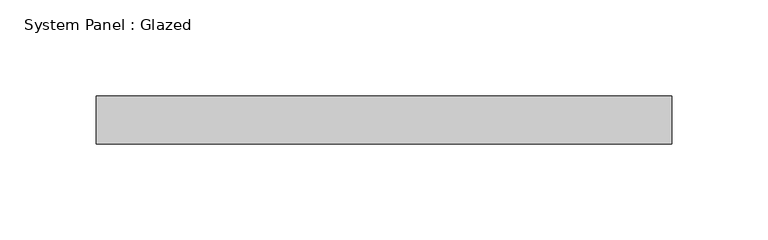
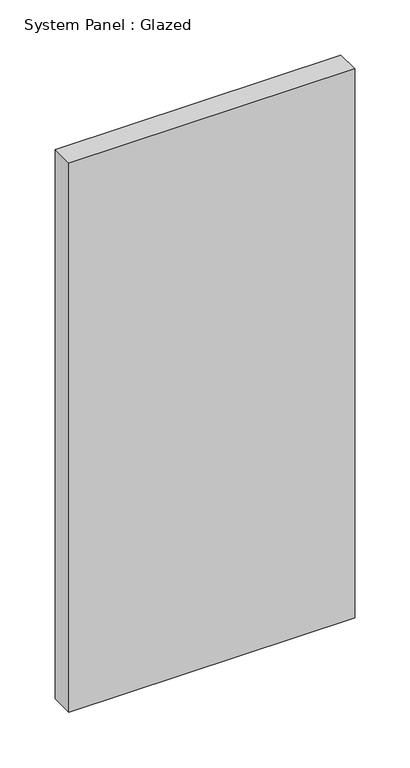
"""IFC4 building model written with IfcOpenShell, lengths in millimetres: plate geometry, System Panel : Glazed."""

from ifc_helpers import new_model, si_unit, origin, origin_with_axes, place, context, project, spatial, polyline, outline, extrude, source, transform, mapped, element, save


def system_panel_glazed_face1e6f(model_context):
    return source(origin(), model_context, "Body", "SweptSolid", [
        extrude(outline(polyline([(149.8911928, 24.5), (-149.8911928, 24.5), (-149.8911928, 49.5), (149.8911928, 49.5), (149.8911928, 24.5)])), origin_with_axes(), (0.0, 0.0, 1.0), 609.6),
    ])


if __name__ == "__main__":
    model = new_model("IFC4")
    model_context = context("Model", 3, world=origin())
    ifc_project = project(units=[si_unit("LENGTHUNIT", "METRE", prefix="MILLI")], contexts=[model_context])
    site = spatial("IfcSite", under=ifc_project)
    building = spatial("IfcBuilding", under=site)
    placement = place(None, origin())
    system_panel_glazed_shape = system_panel_glazed_face1e6f(model_context)
    element("IfcPlate", 1, ObjectType="System Panel : Glazed", at=placement, inside=building, context=model_context, shape_type="MappedRepresentation", body=[
        mapped(system_panel_glazed_shape, transform((0.0, 0.0, 0.0), x_axis=(1.0, 0.0, 0.0), y_axis=(0.0, 1.0, 0.0), z_axis=(0.0, 0.0, 1.0))),
    ])
    save(model, "model.ifc")

# Revit data of these elements
# Type "System Panel : Glazed"
#   Keynote = "H11"
#   Construction Type Id = "GSP4R"
#   Analytic Construction = "1/8 in Pilkington single glazing"
#   Visual Light Transmittance = 0.9
#   Solar Heat Gain Coefficient = 0.86
#   Heat Transfer Coefficient (U) = 6.7069 W/(m²·K)
#   Define Thermal Properties by = 1
# Element 1 (IfcPlate, "System Panel : Glazed")
#   Materials on its faces: "Glass"
# Materials
#   "Glass": class "Glass", colour RGB 0 128 192, transparency 0.9, Description = "Soda Lime Glass", Cost = 0
